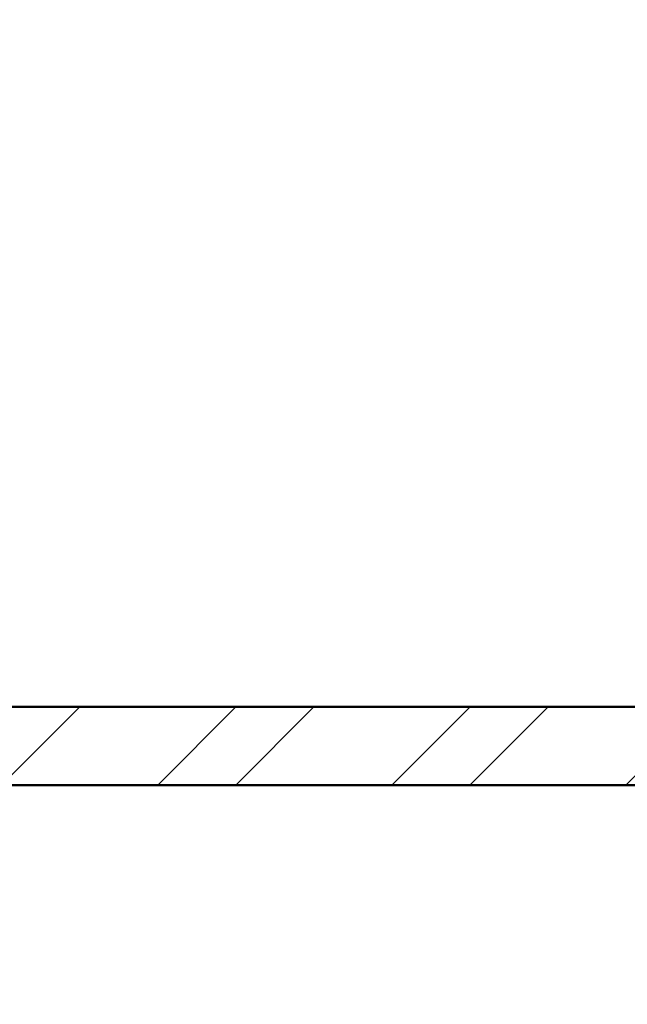
# Model space of a CAD drawing. Units: inches. Extents: x 1901 to 2863, y 888 to 2433.
# Tile 73 of 91: x 2529 to 2564, y 2066 to 2123. Entities that reach past the tile are written whole.
import ezdxf

# ---------------------------------------------------------------- set-up
doc = ezdxf.new("R2010")
doc.units = ezdxf.units.IN
doc.layers.add('A-WALL', color=7, linetype='Continuous', lineweight=50)
doc.layers.add('A-WALL-PATT', color=8, linetype='Continuous', lineweight=13)

msp = doc.modelspace()

# ---------------------------------------------------------------- hatches: boundary and pattern name
at = {"layer": 'A-WALL-PATT'}
h = msp.add_hatch(dxfattribs=at)
h.set_pattern_fill('ANSI32', color=256)
h.paths.add_polyline_path([(2443.926, 2139.888), (2439.426, 2139.888), (2439.426, 2069.348), (2441.676, 2069.348), (2443.926, 2069.348), (2443.926, 2078.634), (2521.926, 2078.634), (2521.926, 2075.067), (2524.176, 2075.067), (2526.426, 2075.067), (2526.426, 2078.634), (2571.755, 2078.634), (2571.755, 2080.884), (2571.755, 2083.134), (2443.926, 2083.134)])
h.paths.add_polyline_path([(2526.426, 2054.634), (2524.176, 2054.634), (2521.926, 2054.634), (2521.926, 2030.634), (2443.926, 2030.634), (2443.926, 2045.348), (2439.426, 2045.348), (2439.426, 1983.867), (2443.926, 1983.867), (2443.926, 2026.134), (2521.926, 2026.134), (2526.426, 2026.134)])
h.paths.add_polyline_path([(2443.926, 1923.867), (2439.426, 1923.867), (2439.426, 1872.634), (2443.926, 1872.634)])
h.paths.add_polyline_path([(2636.233, 1766.134), (2609.926, 1766.134), (2609.926, 1779.785), (2605.426, 1779.785), (2605.426, 1766.134), (2486.614, 1766.134), (2486.614, 1770.671), (2482.114, 1770.671), (2482.114, 1766.134), (2482.114, 1761.634), (2636.233, 1761.634), (2636.233, 1763.884)])
h.paths.add_polyline_path([(2519.536, 1663.384), (2519.536, 1665.634), (2494.926, 1665.634), (2481.831, 1665.634), (2481.831, 1663.384), (2481.831, 1661.134), (2490.426, 1661.134), (2490.426, 1640.157), (2494.926, 1640.157), (2494.926, 1661.134), (2519.536, 1661.134)])
h.paths.add_polyline_path([(2443.926, 1712.134), (2443.926, 1716.634), (2414.464, 1716.634), (2414.464, 1712.134), (2439.426, 1712.134), (2439.426, 1545.507), (2443.926, 1545.507), (2443.926, 1661.134), (2448.475, 1661.134), (2448.475, 1665.634), (2443.926, 1665.634)])
h.paths.add_polyline_path([(2343.426, 1712.134), (2365.525, 1712.134), (2365.525, 1714.384), (2365.525, 1716.634), (2333.871, 1716.634), (2333.871, 1714.384), (2333.871, 1712.134), (2338.926, 1712.134), (2338.926, 1575.634), (2338.926, 1545.507), (2343.426, 1545.507), (2343.426, 1547.507), (2343.426, 1580.134)])
h.paths.add_polyline_path([(2752.926, 1665.634), (2579.536, 1665.634), (2579.536, 1661.134), (2615.926, 1661.134), (2615.926, 1529.134), (2598.931, 1529.134), (2598.931, 1524.634), (2623.127, 1524.634), (2623.127, 1526.884), (2623.127, 1529.134), (2620.426, 1529.134), (2620.426, 1661.134), (2748.426, 1661.134), (2748.426, 1633.499), (2752.926, 1633.499)])
h.paths.add_polyline_path([(2752.926, 1419.929), (2748.426, 1419.929), (2748.426, 1400.134), (2659.426, 1400.134), (2659.426, 1444.333), (2657.176, 1444.333), (2654.926, 1444.333), (2654.926, 1400.134), (2643.649, 1400.134), (2643.649, 1395.634), (2748.426, 1395.634), (2748.426, 1364.035), (2752.926, 1364.035)])
h.paths.add_polyline_path([(2752.926, 1492.878), (2748.426, 1492.878), (2748.426, 1476.634), (2667.426, 1476.634), (2667.426, 1479.71), (2665.176, 1479.71), (2662.926, 1479.71), (2662.926, 1476.634), (2654.926, 1476.634), (2654.926, 1469.536), (2659.426, 1469.536), (2659.426, 1472.134), (2748.426, 1472.134), (2748.426, 1455.929), (2752.926, 1455.929)])
h.paths.add_polyline_path([(2752.926, 1304.035), (2748.426, 1304.035), (2748.426, 1263.634), (2738.66, 1263.634), (2738.66, 1259.134), (2752.926, 1259.134)])
h.paths.add_polyline_path([(2685.926, 1259.134), (2695.49, 1259.134), (2695.49, 1261.384), (2695.49, 1263.634), (2677.837, 1263.634), (2677.837, 1261.384), (2677.837, 1259.134), (2681.426, 1259.134), (2681.426, 1203.634), (2653.277, 1203.634), (2653.277, 1199.134), (2685.926, 1199.134), (2685.926, 1203.634)])
h.paths.add_polyline_path([(2609.426, 1395.634), (2611.848, 1395.634), (2611.848, 1400.134), (2598.888, 1400.134), (2598.888, 1397.884), (2598.888, 1395.634), (2604.926, 1395.634), (2604.926, 1268.134), (2554.726, 1268.134), (2554.726, 1265.884), (2554.726, 1263.634), (2604.926, 1263.634), (2604.926, 1203.634), (2571.306, 1203.634), (2571.306, 1199.134), (2604.926, 1199.134), (2629.277, 1199.134), (2629.277, 1201.384), (2629.277, 1203.634), (2609.426, 1203.634), (2609.426, 1258.634), (2609.426, 1259.134), (2654.804, 1259.134), (2654.804, 1263.634), (2609.426, 1263.634)])
h.paths.add_polyline_path([(2443.926, 1304.035), (2439.426, 1304.035), (2439.426, 1259.134), (2443.926, 1259.134), (2456.16, 1259.134), (2456.16, 1261.384), (2456.16, 1263.634), (2443.926, 1263.634)])
h.paths.add_polyline_path([(2525.426, 1263.634), (2531.778, 1263.634), (2531.778, 1268.134), (2520.926, 1268.134), (2520.926, 1263.634), (2511.409, 1263.634), (2511.409, 1259.134), (2520.926, 1259.134), (2520.926, 1199.134), (2547.306, 1199.134), (2547.306, 1201.384), (2547.306, 1203.634), (2525.426, 1203.634)])
h.paths.add_polyline_path([(2443.926, 1434.842), (2439.426, 1434.842), (2439.426, 1364.035), (2441.676, 1364.035), (2443.926, 1364.035)])
h.paths.add_polyline_path([(2567.134, 1400.134), (2443.926, 1400.134), (2443.926, 1395.634), (2567.134, 1395.634)])
h.paths.add_polyline_path([(2443.926, 1545.507), (2439.426, 1545.507), (2439.426, 1494.842), (2443.926, 1494.842)])
h.paths.add_polyline_path([(2494.926, 1553.349), (2492.676, 1553.349), (2490.426, 1553.349), (2490.426, 1524.634), (2494.926, 1524.634), (2525.936, 1524.634), (2525.936, 1526.884), (2525.936, 1529.134), (2494.926, 1529.134)])
h.paths.add_polyline_path([(2752.926, 1573.499), (2748.426, 1573.499), (2748.426, 1529.134), (2657.759, 1529.134), (2657.759, 1524.634), (2662.926, 1524.634), (2662.926, 1498.631), (2667.426, 1498.631), (2667.426, 1524.634), (2748.426, 1524.634), (2748.426, 1516.878), (2752.926, 1516.878)])
h.paths.add_polyline_path([(2038.602, 2237.418), (2080.174, 2237.418), (2080.174, 2256.075), (2038.602, 2256.075)], flags=9)
h.paths.add_polyline_path([(2292.009, 1062.394), (2539.932, 1062.394), (2539.932, 1099.487), (2292.009, 1099.487)], flags=9)
h.paths.add_polyline_path([(2424.91, 1832.253), (2448.513, 1832.253), (2448.513, 1846.678), (2424.91, 1846.678)], flags=9)
h.paths.add_polyline_path([(2359.076, 1832.253), (2382.678, 1832.253), (2382.678, 1846.678), (2359.076, 1846.678)], flags=9)
h.paths.add_polyline_path([(2352.899, 1684.802), (2367.543, 1684.802), (2367.543, 1697.167), (2352.899, 1697.167)], flags=9)
h.paths.add_polyline_path([(2079.288, 1755.826), (2169.024, 1755.826), (2169.024, 1774.372), (2079.288, 1774.372)], flags=9)
h.paths.add_polyline_path([(2404.09, 1373.857), (2404.09, 1463.593), (2385.544, 1463.593), (2385.544, 1373.857)], flags=9)
h.paths.add_polyline_path([(2268.091, 2236.371), (2309.636, 2236.371), (2309.636, 2255.028), (2268.091, 2255.028)], flags=9)
h.paths.add_polyline_path([(2575.96, 1700.951), (2665.696, 1700.951), (2665.696, 1719.498), (2575.96, 1719.498)], flags=9)
h.paths.add_polyline_path([(2302.962, 1878.474), (2329.524, 1878.474), (2329.524, 1888.777), (2302.962, 1888.777)], flags=9)
h.paths.add_polyline_path([(2097.415, 2240.576), (2126.573, 2240.576), (2126.573, 2259.233), (2097.415, 2259.233)], flags=9)
h.paths.add_polyline_path([(2208.725, 2246.124), (2237.882, 2246.124), (2237.882, 2264.781), (2208.725, 2264.781)], flags=9)
h.paths.add_polyline_path([(2038.147, 1925.958), (2076.987, 1925.958), (2076.987, 1944.615), (2038.147, 1944.615)], flags=9)
h.paths.add_polyline_path([(2239.144, 1926.672), (2288.465, 1926.672), (2288.465, 1945.329), (2239.144, 1945.329)], flags=9)
h.paths.add_polyline_path([(2175.429, 2007.33), (2212.356, 2007.33), (2212.356, 2025.987), (2175.429, 2025.987)], flags=9)
h.paths.add_polyline_path([(2225.034, 2091.794), (2263.875, 2091.794), (2263.875, 2110.451), (2225.034, 2110.451)], flags=9)
h.paths.add_polyline_path([(2035.398, 2098.478), (2074.238, 2098.478), (2074.238, 2117.135), (2035.398, 2117.135)], flags=9)
h.paths.add_polyline_path([(2050.102, 2029.209), (2083.26, 2029.209), (2083.26, 2047.866), (2050.102, 2047.866)], flags=9)
h.paths.add_polyline_path([(2069.677, 1956.719), (2098.835, 1956.719), (2098.835, 1975.376), (2069.677, 1975.376)], flags=9)
h.paths.add_polyline_path([(2328.62, 1753.336), (2361.663, 1753.336), (2361.663, 1771.993), (2328.62, 1771.993)], flags=9)
h.paths.add_polyline_path([(2395.162, 2060.888), (2395.162, 2140.654), (2378.676, 2140.654), (2378.676, 2060.888)], flags=9)
h.paths.add_polyline_path([(2463.728, 2059.02), (2492.886, 2059.02), (2492.886, 2077.677), (2463.728, 2077.677)], flags=9)
h.paths.add_polyline_path([(2458.027, 2181.536), (2496.868, 2181.536), (2496.868, 2200.194), (2458.027, 2200.194)], flags=9)
h.paths.add_polyline_path([(2456.855, 2228.831), (2498.401, 2228.831), (2498.401, 2247.488), (2456.855, 2247.488)], flags=9)
h.paths.add_polyline_path([(2527.577, 2243.074), (2556.735, 2243.074), (2556.735, 2261.731), (2527.577, 2261.731)], flags=9)
h.paths.add_polyline_path([(2694.461, 2232.767), (2736.033, 2232.767), (2736.033, 2251.425), (2694.461, 2251.425)], flags=9)
h.paths.add_polyline_path([(2637.821, 2249.225), (2666.979, 2249.225), (2666.979, 2267.882), (2637.821, 2267.882)], flags=9)
h.paths.add_polyline_path([(2623.687, 2183.541), (2662.528, 2183.541), (2662.528, 2202.199), (2623.687, 2202.199)], flags=9)
h.paths.add_polyline_path([(2691.965, 2021.5), (2725.124, 2021.5), (2725.124, 2040.157), (2691.965, 2040.157)], flags=9)
h.paths.add_polyline_path([(2621.043, 1975.912), (2662.335, 1975.912), (2662.335, 1994.569), (2621.043, 1994.569)], flags=9)
h.paths.add_polyline_path([(2479.032, 1927.62), (2519.844, 1927.62), (2519.844, 1946.277), (2479.032, 1946.277)], flags=9)
h.paths.add_polyline_path([(2670.941, 1849.076), (2716.005, 1849.076), (2716.005, 1867.734), (2670.941, 1867.734)], flags=9)
h.paths.add_polyline_path([(2523.613, 1782.956), (2550.175, 1782.956), (2550.175, 1793.26), (2523.613, 1793.26)], flags=9)
h.paths.add_polyline_path([(2450.841, 1207.331), (2492.386, 1207.331), (2492.386, 1225.989), (2450.841, 1225.989)], flags=9)
h.paths.add_polyline_path([(2527.751, 1203.841), (2556.908, 1203.841), (2556.908, 1222.499), (2527.751, 1222.499)], flags=9)
h.paths.add_polyline_path([(2639.111, 1207.2), (2668.268, 1207.2), (2668.268, 1225.857), (2639.111, 1225.857)], flags=9)
h.paths.add_polyline_path([(2692.594, 1218.965), (2734.167, 1218.965), (2734.167, 1237.623), (2692.594, 1237.623)], flags=9)
h.paths.add_polyline_path([(2669.266, 1366.329), (2708.106, 1366.329), (2708.106, 1384.987), (2669.266, 1384.987)], flags=25)
h.paths.add_polyline_path([(2463.313, 1358.031), (2502.153, 1358.031), (2502.153, 1376.688), (2463.313, 1376.688)], flags=9)
h.paths.add_polyline_path([(2494.725, 1449.963), (2531.652, 1449.963), (2531.652, 1468.62), (2494.725, 1468.62)], flags=9)
h.paths.add_polyline_path([(2675.565, 1422.157), (2708.724, 1422.157), (2708.724, 1440.815), (2675.565, 1440.815)], flags=25)
h.paths.add_polyline_path([(2685.634, 1493.891), (2714.792, 1493.891), (2714.792, 1512.548), (2685.634, 1512.548)], flags=9)
h.paths.add_polyline_path([(2686.805, 1529.913), (2725.645, 1529.913), (2725.645, 1548.57), (2686.805, 1548.57)], flags=25)
h.paths.add_polyline_path([(2503.651, 1537.991), (2552.972, 1537.991), (2552.972, 1556.648), (2503.651, 1556.648)], flags=9)
h.paths.add_polyline_path([(2291.713, 1643.504), (2318.275, 1643.504), (2318.275, 1653.807), (2291.713, 1653.807)], flags=9)
h.paths.add_polyline_path([(2450.626, 1610.52), (2477.189, 1610.52), (2477.189, 1620.824), (2450.626, 1620.824)], flags=9)
h.paths.add_polyline_path([(2359.985, 1551.814), (2422.253, 1551.814), (2422.253, 1562.117), (2359.985, 1562.117)], flags=9)
h.paths.add_polyline_path([(2280.106, 1249.006), (2321.651, 1249.006), (2321.651, 1267.663), (2280.106, 1267.663)], flags=9)
h.paths.add_polyline_path([(2164.057, 1274.232), (2193.215, 1274.232), (2193.215, 1292.889), (2164.057, 1292.889)], flags=9)
h.paths.add_polyline_path([(2118.21, 1277.694), (2151.252, 1277.694), (2151.252, 1296.351), (2118.21, 1296.351)], flags=9)
h.paths.add_polyline_path([(2031.946, 1268.529), (2073.519, 1268.529), (2073.519, 1287.187), (2031.946, 1287.187)], flags=9)
h.paths.add_polyline_path([(2050.199, 1409.079), (2089.04, 1409.079), (2089.04, 1427.736), (2050.199, 1427.736)], flags=9)
h.paths.add_polyline_path([(2243.743, 1421.032), (2282.584, 1421.032), (2282.584, 1439.689), (2243.743, 1439.689)], flags=9)
h.paths.add_polyline_path([(2190.746, 1509.769), (2231.558, 1509.769), (2231.558, 1528.426), (2190.746, 1528.426)], flags=9)
h.paths.add_polyline_path([(2058.392, 1475.415), (2091.55, 1475.415), (2091.55, 1494.073), (2058.392, 1494.073)], flags=9)
h.paths.add_polyline_path([(2062.447, 1553.09), (2091.605, 1553.09), (2091.605, 1571.747), (2062.447, 1571.747)], flags=9)
h.paths.add_polyline_path([(2219.524, 1590.365), (2266.147, 1590.365), (2266.147, 1609.022), (2219.524, 1609.022)], flags=9)
h.paths.add_polyline_path([(2041.072, 1584.188), (2079.912, 1584.188), (2079.912, 1602.845), (2041.072, 1602.845)], flags=9)

# ---------------------------------------------------------------- linework, layer by layer
at = {"layer": 'A-WALL'}
for p, q in [((2443.926, 2083.134), (2573.051, 2083.134)), ((2526.426, 2078.634), (2571.755, 2078.634))]:
    msp.add_line(p, q, dxfattribs=at)

doc.saveas('drawing.dxf')
